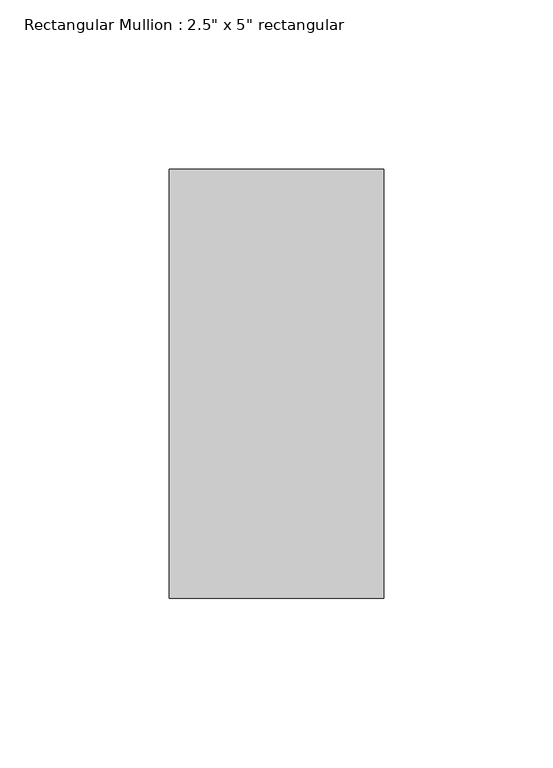
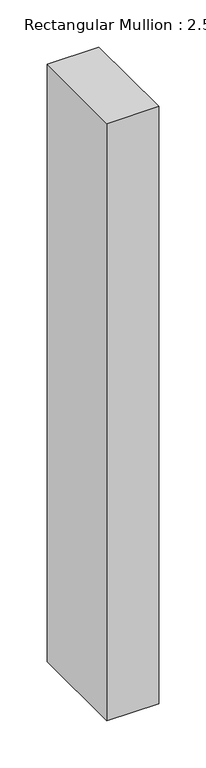
"""IFC4 building model written with IfcOpenShell, lengths in millimetres: member geometry."""

from ifc_helpers import new_model, si_unit, frame, origin, place, context, project, spatial, polyline, outline, extrude, source, transform, mapped, element, save


def member_c1a40fae(model_context):
    return source(origin(), model_context, "Body", "SweptSolid", [
        extrude(outline(polyline([(0.0, 63.5), (0.0, -63.5), (-63.5, -63.5), (-63.5, 63.5), (0.0, 63.5)])), frame((0.0, 0.0, -774.2920746), z_axis=(0.0, 0.0, 1.0), x_axis=(1.0, 0.0, 0.0)), (0.0, 0.0, 1.0), 774.2920746),
    ])


if __name__ == "__main__":
    model = new_model("IFC4")
    model_context = context("Model", 3, world=origin())
    ifc_project = project(units=[si_unit("LENGTHUNIT", "METRE", prefix="MILLI")], contexts=[model_context])
    site = spatial("IfcSite", under=ifc_project)
    building = spatial("IfcBuilding", under=site)
    placement = place(None, origin())
    member_shape = member_c1a40fae(model_context)
    element("IfcMember", 1, ObjectType="Rectangular Mullion : 2.5\" x 5\" rectangular", at=placement, inside=building, context=model_context, shape_type="MappedRepresentation", body=[
        mapped(member_shape, transform((0.0, 0.0, 0.0), x_axis=(1.0, 0.0, 0.0), y_axis=(0.0, 1.0, 0.0), z_axis=(0.0, 0.0, 1.0))),
    ])
    save(model, "model.ifc")

# Revit data of these elements
# Type "Rectangular Mullion : 2.5\" x 5\" rectangular"
#   built-in parameter 1007304 = 0.416667 (stored number, unit not read)
#   built-in parameter 1007301 = 0.104167 (stored number, unit not read)
#   built-in parameter 1007300 = 0.104167 (stored number, unit not read)
# Element 1 (IfcMember, "Rectangular Mullion : 2.5\" x 5\" rectangular")
#   Materials on its faces: "Aluminum"
# Materials
#   "Aluminum": class "Metal", colour RGB 247 247 247, transparency 0, Description = "Aluminum 6061", Cost = 0
